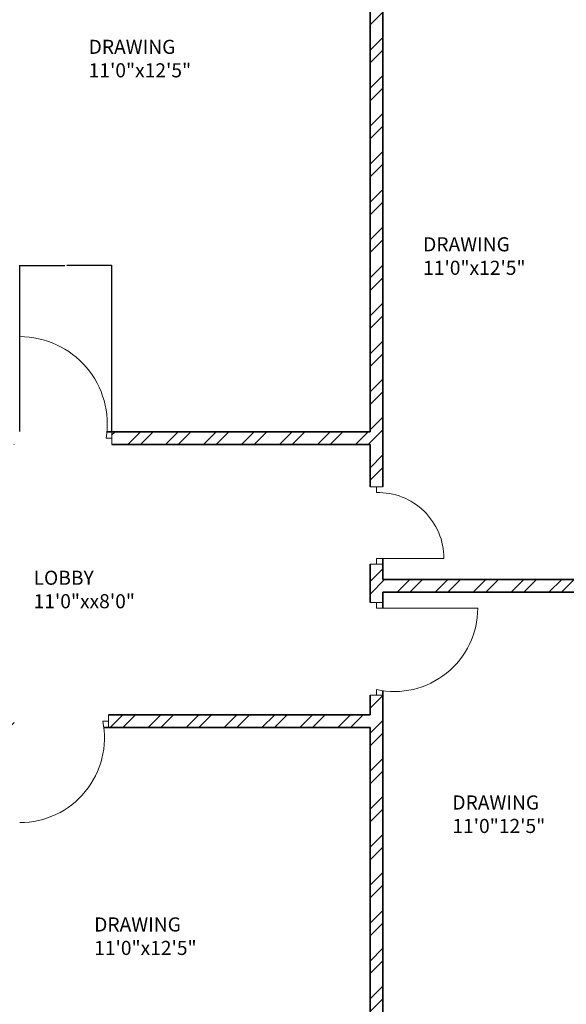
# Model space of a CAD drawing. Units: inches. Extents: x 1962 to 2771, y 1245 to 2660.
# Tile 60 of 114: x 2247 to 2441, y 1831 to 2180. Entities that reach past the tile are written whole.
import ezdxf

# ---------------------------------------------------------------- set-up
doc = ezdxf.new("R2010")
doc.units = ezdxf.units.IN
for name, color, linetype, lineweight in [('A-ANNO-DIMS', 2, 'Continuous', 18), ('A-AREA-IDEN', 7, 'Continuous', 18), ('A-DOOR', 3, 'Continuous', 18), ('A-WALL', 7, 'Continuous', 35), ('A-WALL-PATT', 252, 'Continuous', 13)]:
    doc.layers.add(name, color=color, linetype=linetype, lineweight=lineweight)
doc.styles.get("Standard").update_dxf_attribs({"font": 'arial.ttf'})
doc.dimstyles.get("Standard").update_dxf_attribs({"dimtxt": 0.18, "dimasz": 0.18, "dimexe": 0.18, "dimexo": 0.0625, "dimgap": 0.09, "dimtad": 0, "dimtih": 1, "dimtoh": 1, "dimdec": 4, "dimzin": 0, "dimdsep": 46, "dimtxsty": 'Standard', "dimcen": 0.09, "dimadec": 0, "dimazin": 0, "dimtfac": 1, "dimtdec": 4, "dimtofl": 0, "dimtmove": 0, "dimatfit": 3, "dimfxl": 1, "dimtolj": 1, "dimtzin": 0, "dimarcsym": 0})

# ---------------------------------------------------------------- blocks, each defined once
blk = doc.blocks.new('*D40')
at = {"layer": 'A-ANNO-DIMS', "color": 0, "lineweight": -2, "transparency": 16777216}
for p, q in [((2072.02, 2033.91), (2072.02, 2583.47)), ((2072.2, 2583.29), (2366.02, 2583.29)), ((2660.63, 2583.29), (2366.81, 2583.29)), ((2660.81, 2524.41), (2660.81, 2583.47))]:
    blk.add_line(p, q, dxfattribs=at)
at = {"layer": 'A-ANNO-DIMS', "color": 0, "transparency": 16777216}
for points in [[(2072.2, 2583.32), (2072.2, 2583.26), (2072.02, 2583.29)], [(2660.63, 2583.32), (2660.63, 2583.26), (2660.81, 2583.29)]]:
    blk.add_solid(points, dxfattribs=at)
at = {"layer": 'Defpoints', "color": 0, "transparency": 16777216}
for p in [(2660.81, 2583.29), (2660.81, 2524.34), (2072.02, 2033.84)]:
    blk.add_point(p, dxfattribs=at)
at = {"layer": 'A-ANNO-DIMS', "color": 0, "transparency": 16777216, "insert": (2366.41, 2583.29), "char_height": 0.18, "attachment_point": 5}
blk.add_mtext('\\A1;588.8', dxfattribs=at)
blk = doc.blocks.new('*D45')
at = {"layer": 'A-ANNO-DIMS', "color": 0, "lineweight": -2, "transparency": 16777216}
for p, q in [((2246.94, 2033.91), (2246.94, 2092.97)), ((2247.12, 2092.79), (2262.91, 2092.79)), ((2279.48, 2092.79), (2263.69, 2092.79)), ((2279.66, 2033.91), (2279.66, 2092.97))]:
    blk.add_line(p, q, dxfattribs=at)
at = {"layer": 'A-ANNO-DIMS', "color": 0, "transparency": 16777216}
for points in [[(2247.12, 2092.82), (2247.12, 2092.76), (2246.94, 2092.79)], [(2279.48, 2092.82), (2279.48, 2092.76), (2279.66, 2092.79)]]:
    blk.add_solid(points, dxfattribs=at)
at = {"layer": 'Defpoints', "color": 0, "transparency": 16777216}
for p in [(2279.66, 2092.79), (2246.94, 2033.84), (2279.66, 2033.84)]:
    blk.add_point(p, dxfattribs=at)
at = {"layer": 'A-ANNO-DIMS', "color": 0, "transparency": 16777216, "insert": (2263.3, 2092.79), "char_height": 0.18, "attachment_point": 5}
blk.add_mtext('\\A1;32.72', dxfattribs=at)

msp = doc.modelspace()

# ---------------------------------------------------------------- hatches: boundary and pattern name
at = {"layer": 'A-WALL-PATT'}
h = msp.add_hatch(dxfattribs=at)
h.set_pattern_fill('ANSI32', color=256)
h.paths.add_polyline_path([(2090.8074, 2467.3437), (2141.6481, 2467.3437), (2141.6481, 2469.5937), (2141.6481, 2471.8437), (2086.3074, 2471.8437), (2086.3074, 2422.5333), (2090.8074, 2422.5333)])
h.paths.add_polyline_path([(2282.7664, 2471.8437), (2204.8982, 2471.8437), (2204.8982, 2467.3437), (2234.8074, 2467.3437), (2234.8074, 2311.3437), (2228.7492, 2311.3437), (2228.7492, 2306.8437), (2234.8074, 2306.8437), (2331.9227, 2306.8437), (2331.9227, 2309.0937), (2331.9227, 2311.3437), (2239.3074, 2311.3437), (2239.3074, 2467.3437), (2282.7664, 2467.3437), (2282.7664, 2469.5937)])
h.paths.add_polyline_path([(2471.4531, 2519.8437), (2552.011, 2519.8437), (2564.3996, 2519.8437), (2564.3996, 2511.1389), (2568.8996, 2511.1389), (2568.8996, 2524.3437), (2466.9531, 2524.3437), (2466.9531, 2471.8437), (2450.0749, 2471.8437), (2446.4672, 2471.8437), (2446.4672, 2467.3437), (2450.0749, 2467.3437), (2475.9988, 2467.3437), (2475.9988, 2469.5937), (2475.9988, 2471.8437), (2471.4531, 2471.8437)])
h.paths.add_polyline_path([(2575.2231, 2469.5937), (2575.2231, 2471.8437), (2568.8996, 2471.8437), (2568.8996, 2487.1389), (2564.3996, 2487.1389), (2564.3996, 2471.8437), (2556.511, 2471.8437), (2499.2904, 2471.8437), (2499.2904, 2467.3437), (2507.8074, 2467.3437), (2507.8074, 2311.3437), (2414.863, 2311.3437), (2414.863, 2306.8437), (2512.3074, 2306.8437), (2517.0114, 2306.8437), (2517.0114, 2309.0937), (2517.0114, 2311.3437), (2512.3074, 2311.3437), (2512.3074, 2467.3437), (2575.2231, 2467.3437)])
h.paths.add_polyline_path([(2660.8074, 2471.8437), (2600.9602, 2471.8437), (2600.9602, 2467.3437), (2656.3074, 2467.3437), (2656.3074, 2432.5704), (2660.8074, 2432.5704)])
h.paths.add_polyline_path([(2660.8074, 2372.5704), (2656.3074, 2372.5704), (2656.3074, 2311.3437), (2600.276, 2311.3437), (2600.276, 2309.0937), (2600.276, 2306.8437), (2656.3074, 2306.8437), (2656.3074, 2296.2593), (2660.8074, 2296.2593)])
h.paths.add_polyline_path([(2572.3074, 2306.8437), (2577.1385, 2306.8437), (2577.1385, 2311.3437), (2551.082, 2311.3437), (2551.082, 2306.8437), (2567.8074, 2306.8437), (2567.8074, 2258.8437), (2540.0574, 2258.8437), (2540.0574, 2256.5937), (2540.0574, 2254.3437), (2567.8074, 2254.3437), (2656.3074, 2254.3437), (2656.3074, 2236.9085), (2660.8074, 2236.9085), (2660.8074, 2272.2593), (2656.3074, 2272.2593), (2656.3074, 2258.8437), (2572.3074, 2258.8437)])
h.paths.add_polyline_path([(2512.3074, 2254.3437), (2518.8716, 2254.3437), (2518.8716, 2256.5937), (2518.8716, 2258.8437), (2507.8074, 2258.8437), (2507.8074, 2177.8437), (2567.8074, 2177.8437), (2567.8074, 2172.9628), (2572.3074, 2172.9628), (2572.3074, 2177.8437), (2656.3074, 2177.8437), (2656.3074, 2166.4846), (2660.8074, 2166.4846), (2660.8074, 2200.9085), (2656.3074, 2200.9085), (2656.3074, 2182.3437), (2512.3074, 2182.3437)])
h.paths.add_polyline_path([(2656.3074, 2129.8437), (2572.3074, 2129.8437), (2572.3074, 2150.3044), (2570.0574, 2150.3044), (2567.8074, 2150.3044), (2567.8074, 2129.8437), (2507.8074, 2129.8437), (2507.8074, 2116.3027), (2510.0574, 2116.3027), (2512.3074, 2116.3027), (2512.3074, 2125.3437), (2567.8074, 2125.3437), (2572.3074, 2125.3437), (2656.3074, 2125.3437)])
h.paths.add_polyline_path([(2090.8074, 2362.5333), (2086.3074, 2362.5333), (2086.3074, 2298.6242), (2090.8074, 2298.6242), (2090.8074, 2306.8437), (2174.8074, 2306.8437), (2174.8074, 2286.4178), (2179.3074, 2286.4178), (2179.3074, 2306.8437), (2192.8641, 2306.8437), (2192.8641, 2309.0937), (2192.8641, 2311.3437), (2090.8074, 2311.3437)])
h.paths.add_polyline_path([(2209.156, 2258.8437), (2179.3074, 2258.8437), (2179.3074, 2263.2236), (2177.0574, 2263.2236), (2174.8074, 2263.2236), (2174.8074, 2258.8437), (2090.8074, 2258.8437), (2090.8074, 2274.6242), (2086.3074, 2274.6242), (2086.3074, 2238.2967), (2088.5574, 2238.2967), (2090.8074, 2238.2967), (2090.8074, 2254.3437), (2209.156, 2254.3437)])
h.paths.add_polyline_path([(2090.8074, 2177.8437), (2234.8074, 2177.8437), (2234.8074, 2173.1428), (2239.3074, 2173.1428), (2239.3074, 2258.8437), (2230.8442, 2258.8437), (2230.8442, 2256.5937), (2230.8442, 2254.3437), (2234.8074, 2254.3437), (2234.8074, 2182.3437), (2090.8074, 2182.3437), (2090.8074, 2202.2967), (2086.3074, 2202.2967), (2086.3074, 2140.0389), (2090.8074, 2140.0389)])
h.paths.add_polyline_path([(2090.8074, 2080.0389), (2086.3074, 2080.0389), (2086.3074, 2033.8437), (2090.8074, 2033.8437)], flags=17)
h.paths.add_polyline_path([(2244.9405, 2033.8437), (2239.3074, 2033.8437), (2239.3074, 2142.0665), (2237.2592, 2142.0665), (2234.8074, 2142.0665), (2234.8074, 2033.8437), (2090.8074, 2033.8437), (2076.5204, 2033.8437), (2072.0204, 2033.8437), (2072.0204, 2000.4493), (2076.5204, 2000.4493), (2076.5204, 2029.3437), (2090.8074, 2029.3437), (2244.9405, 2029.3437), (2244.9405, 2031.5937)])
h.paths.add_polyline_path([(2234.8074, 1933.3437), (2076.5204, 1933.3437), (2076.5204, 1952.4493), (2074.2704, 1952.4493), (2072.0204, 1952.4493), (2072.0204, 1933.3437), (2072.0204, 1928.8437), (2234.8074, 1928.8437)])
h.paths.add_polyline_path([(2090.8074, 1928.8437), (2086.3074, 1928.8437), (2086.3074, 1906.5013), (2090.8074, 1906.5013)])
h.paths.add_polyline_path([(2090.8074, 1846.5013), (2086.3074, 1846.5013), (2086.3074, 1769.9917), (2088.5574, 1769.9917), (2090.8074, 1769.9917), (2090.8074, 1780.3437), (2234.8074, 1780.3437), (2234.8074, 1708.3437), (2230.3764, 1708.3437), (2230.3764, 1703.8437), (2239.3074, 1703.8437), (2239.3074, 1792.6669), (2237.0574, 1792.6669), (2234.8074, 1792.6669), (2234.8074, 1784.8437), (2090.8074, 1784.8437)])
h.paths.add_polyline_path([(2239.3074, 1928.8437), (2244.9405, 1928.8437), (2244.9405, 1931.0937), (2244.9405, 1933.3437), (2234.8074, 1933.3437), (2234.8074, 1928.8437), (2234.8074, 1825.5949), (2239.3074, 1825.5949)])
h.paths.add_polyline_path([(2148.0425, 1649.0937), (2148.0425, 1651.3437), (2090.8074, 1651.3437), (2090.8074, 1646.8437), (2148.0425, 1646.8437)], flags=0)
h.paths.add_polyline_path([(2207.5601, 1708.3437), (2090.8074, 1708.3437), (2090.8074, 1703.8437), (2174.8074, 1703.8437), (2174.8074, 1651.3437), (2170.4457, 1651.3437), (2170.4457, 1646.8437), (2195.9924, 1646.8437), (2195.9924, 1649.0937), (2195.9924, 1651.3437), (2179.3074, 1651.3437), (2179.3074, 1703.8437), (2207.5601, 1703.8437), (2207.5601, 1706.0937)])
h.paths.add_polyline_path([(2090.8074, 1733.9917), (2086.3074, 1733.9917), (2086.3074, 1696.1032), (2088.5574, 1696.1032), (2090.8074, 1696.1032)])
h.paths.add_polyline_path([(2090.8074, 1672.1032), (2086.3074, 1672.1032), (2086.3074, 1600.3335), (2090.8074, 1600.3335)])
h.paths.add_polyline_path([(2090.8074, 1540.3335), (2086.3074, 1540.3335), (2086.3074, 1486.3437), (2139.6766, 1486.3437), (2139.6766, 1490.8437), (2090.8074, 1490.8437)])
h.paths.add_polyline_path([(2302.3876, 1490.8437), (2239.3074, 1490.8437), (2239.3074, 1646.8437), (2335.9994, 1646.8437), (2335.9994, 1651.3437), (2229.884, 1651.3437), (2229.884, 1646.8437), (2234.8074, 1646.8437), (2234.8074, 1490.8437), (2202.7103, 1490.8437), (2202.7103, 1488.5937), (2202.7103, 1486.3437), (2275.0699, 1486.3437), (2275.0699, 1475.772), (2279.5699, 1475.772), (2279.5699, 1486.3437), (2302.3876, 1486.3437)])
h.paths.add_polyline_path([(2279.5699, 1451.772), (2275.0699, 1451.772), (2275.0699, 1438.3437), (2174.8074, 1438.3437), (2174.8074, 1486.3437), (2179.7922, 1486.3437), (2179.7922, 1490.8437), (2163.3585, 1490.8437), (2163.3585, 1488.5937), (2163.3585, 1486.3437), (2170.3074, 1486.3437), (2170.3074, 1433.8437), (2279.5699, 1433.8437)])
h.paths.add_polyline_path([(2427.2363, 1490.8437), (2375.8074, 1490.8437), (2375.8074, 1646.8437), (2381.6401, 1646.8437), (2381.6401, 1651.3437), (2365.887, 1651.3437), (2365.887, 1649.0937), (2365.887, 1646.8437), (2371.3074, 1646.8437), (2371.3074, 1490.8437), (2327.5627, 1490.8437), (2327.5627, 1488.5937), (2327.5627, 1486.3437), (2371.3074, 1486.3437), (2371.3074, 1433.8437), (2375.8074, 1433.8437), (2375.8074, 1486.3437), (2427.2363, 1486.3437)])
h.paths.add_polyline_path([(2512.3074, 1646.8437), (2519.4351, 1646.8437), (2519.4351, 1649.0937), (2519.4351, 1651.3437), (2507.8074, 1651.3437), (2416.0063, 1651.3437), (2416.0063, 1649.0937), (2416.0063, 1646.8437), (2507.8074, 1646.8437), (2507.8074, 1490.8437), (2497.0532, 1490.8437), (2497.0532, 1488.5937), (2497.0532, 1486.3437), (2574.9344, 1486.3437), (2574.9344, 1476.0181), (2579.4344, 1476.0181), (2579.4344, 1486.3437), (2584.4872, 1486.3437), (2584.3074, 1490.8437), (2512.3074, 1490.8437)])
h.paths.add_polyline_path([(2470.5091, 1486.3437), (2473.9767, 1486.3437), (2473.9767, 1490.8437), (2449.6605, 1490.8437), (2449.6605, 1488.5937), (2449.6605, 1486.3437), (2466.0091, 1486.3437), (2466.0091, 1433.8437), (2470.5091, 1433.8437), (2579.4344, 1433.8437), (2579.4344, 1452.0181), (2574.9344, 1452.0181), (2574.9344, 1438.3437), (2554.5091, 1438.3437), (2470.5091, 1438.3437)])
h.paths.add_polyline_path([(2656.3074, 1490.8437), (2611.86, 1490.8437), (2611.86, 1486.3437), (2656.3074, 1486.3437)])
h.paths.add_polyline_path([(2660.8074, 1532.7007), (2658.5574, 1532.7007), (2656.3074, 1532.7007), (2656.3074, 1486.3437), (2660.8074, 1486.3437)])
h.paths.add_polyline_path([(2660.8074, 1664.9663), (2656.3074, 1664.9663), (2656.3074, 1651.3437), (2602.2313, 1651.3437), (2602.2313, 1646.8437), (2656.3074, 1646.8437), (2656.3074, 1592.7007), (2660.8074, 1592.7007)])
h.paths.add_polyline_path([(2660.8074, 1724.5221), (2656.3074, 1724.5221), (2656.3074, 1703.8437), (2542.4725, 1703.8437), (2542.4725, 1699.3437), (2567.8074, 1699.3437), (2567.8074, 1651.3437), (2552.7766, 1651.3437), (2552.7766, 1649.0937), (2552.7766, 1646.8437), (2577.2878, 1646.8437), (2577.2878, 1649.0937), (2577.2878, 1651.3437), (2572.3074, 1651.3437), (2572.3074, 1699.3437), (2656.3074, 1699.3437), (2656.3074, 1688.9663), (2660.8074, 1688.9663)])
h.paths.add_polyline_path([(2660.8074, 1880.6524), (2656.3074, 1880.6524), (2656.3074, 1832.8437), (2512.3074, 1832.8437), (2512.3074, 1837.8959), (2507.8074, 1837.8959), (2507.8074, 1828.3437), (2567.8074, 1828.3437), (2567.8074, 1804.3437), (2572.3074, 1804.3437), (2572.3074, 1828.3437), (2656.3074, 1828.3437), (2656.3074, 1818.6778), (2660.8074, 1818.6778)])
h.paths.add_polyline_path([(2660.8074, 1794.6778), (2656.3074, 1794.6778), (2656.3074, 1780.3437), (2572.3074, 1780.3437), (2572.3074, 1783.0303), (2570.0574, 1783.0303), (2567.8074, 1783.0303), (2567.8074, 1780.3437), (2507.8074, 1780.3437), (2507.8074, 1699.3437), (2517.8858, 1699.3437), (2517.8858, 1701.5937), (2517.8858, 1703.8437), (2512.3074, 1703.8437), (2512.3074, 1775.8437), (2656.3074, 1775.8437), (2656.3074, 1760.5221), (2660.8074, 1760.5221)])
h.paths.add_polyline_path([(2660.8074, 1981.3437), (2660.8074, 2020.2808), (2658.5574, 2020.2808), (2656.3074, 2020.2808), (2656.3074, 1981.3437), (2512.3074, 1981.3437), (2512.3074, 2086.6996), (2507.8074, 2086.6996), (2507.8074, 1981.3437), (2375.8074, 1981.3437), (2375.8074, 1986.8505), (2373.5574, 1986.8505), (2371.3074, 1986.8505), (2371.3074, 1973.2607), (2375.8074, 1973.2607), (2375.8074, 1976.8437), (2507.8074, 1976.8437), (2507.8074, 1865.4281), (2510.0574, 1865.4281), (2512.3074, 1865.4281), (2512.3074, 1976.8437), (2660.8074, 1976.8437)])
h.paths.add_polyline_path([(2375.8074, 1940.297), (2373.5574, 1940.297), (2371.3074, 1940.297), (2371.3074, 1933.3437), (2278.4434, 1933.3437), (2278.4434, 1928.8437), (2371.3074, 1928.8437), (2371.3074, 1651.3437), (2375.8074, 1651.3437)])
h.paths.add_polyline_path([(2660.8074, 1976.8437), (2656.3074, 1976.8437), (2656.3074, 1940.6524), (2660.8074, 1940.6524)], flags=17)
h.paths.add_polyline_path([(2660.8074, 2142.4846), (2656.3074, 2142.4846), (2656.3074, 2080.2808), (2660.8074, 2080.2808)])
h.paths.add_polyline_path([(2381.4189, 2311.3437), (2375.8074, 2311.3437), (2375.8074, 2467.3437), (2424.7242, 2467.3437), (2424.7242, 2469.5937), (2424.7242, 2471.8437), (2375.8074, 2471.8437), (2375.8074, 2524.3437), (2371.3074, 2524.3437), (2371.3074, 2471.8437), (2307.2097, 2471.8437), (2307.2097, 2467.3437), (2371.3074, 2467.3437), (2371.3074, 2311.3437), (2366.8901, 2311.3437), (2366.8901, 2306.8437), (2371.3074, 2306.8437), (2371.3074, 2033.8437), (2279.6589, 2033.8437), (2279.6589, 2029.3437), (2371.3074, 2029.3437), (2371.3074, 2014.2598), (2375.8074, 2014.2598), (2375.8074, 2306.8437), (2381.4189, 2306.8437)])
h.paths.add_polyline_path([(2263.3074, 2524.3437), (2170.3074, 2524.3437), (2170.3074, 2519.8437), (2170.3074, 2471.8437), (2165.0312, 2471.8437), (2165.0312, 2467.3437), (2179.6721, 2467.3437), (2179.6721, 2469.5161), (2179.6721, 2471.8437), (2174.8074, 2471.8437), (2174.8074, 2519.8437), (2258.8074, 2519.8437), (2258.8074, 2511.6436), (2263.3074, 2511.6436)])
h.paths.add_polyline_path([(2245.0232, 1361.4123), (2492.9468, 1361.4123), (2492.9468, 1398.505), (2245.0232, 1398.505)], flags=9)
h.paths.add_polyline_path([(2388.1434, 2086.6936), (2425.0704, 2086.6936), (2425.0704, 2105.3509), (2388.1434, 2105.3509)], flags=9)
h.paths.add_polyline_path([(2404.922, 2242.6744), (2445.7337, 2242.6744), (2445.7337, 2261.3318), (2404.922, 2261.3318)], flags=9)
h.paths.add_polyline_path([(2269.4107, 2156.7935), (2306.3378, 2156.7935), (2306.3378, 2175.4508), (2269.4107, 2175.4508)], flags=9)
h.paths.add_polyline_path([(2269.3277, 2233.4343), (2306.2547, 2233.4343), (2306.2547, 2252.0917), (2269.3277, 2252.0917)], flags=9)
h.paths.add_polyline_path([(2431.6052, 2320.6922), (2470.4456, 2320.6922), (2470.4456, 2339.3495), (2431.6052, 2339.3495)], flags=25)
h.paths.add_polyline_path([(2249.6902, 2315.7608), (2288.5306, 2315.7608), (2288.5306, 2334.4182), (2249.6902, 2334.4182)], flags=25)
h.paths.add_polyline_path([(2096.9301, 2314.3181), (2135.7704, 2314.3181), (2135.7704, 2332.9755), (2096.9301, 2332.9755)], flags=25)
h.paths.add_polyline_path([(2134.3475, 2285.7089), (2161.4655, 2285.7089), (2161.4655, 2304.3662), (2134.3475, 2304.3662)], flags=9)
h.paths.add_polyline_path([(2126.5155, 2209.4076), (2159.9227, 2209.4076), (2159.9227, 2228.065), (2126.5155, 2228.065)], flags=25)
h.paths.add_polyline_path([(2110.5753, 2141.5299), (2149.4157, 2141.5299), (2149.4157, 2160.1872), (2110.5753, 2160.1872)], flags=25)
h.paths.add_polyline_path([(2249.8618, 1968.3317), (2286.3966, 1968.3317), (2286.3966, 1986.989), (2249.8618, 1986.989)], flags=9)
h.paths.add_polyline_path([(2395.9507, 1777.0051), (2436.7624, 1777.0051), (2436.7624, 1795.6625), (2395.9507, 1795.6625)], flags=9)
h.paths.add_polyline_path([(2398.5259, 1888.5651), (2435.0062, 1888.5651), (2435.0062, 1907.2224), (2398.5259, 1907.2224)], flags=25)
h.paths.add_polyline_path([(2259.3506, 1728.3559), (2296.2776, 1728.3559), (2296.2776, 1747.0132), (2259.3506, 1747.0132)], flags=9)
h.paths.add_polyline_path([(2271.3698, 1845.268), (2308.2968, 1845.268), (2308.2968, 1863.9253), (2271.3698, 1863.9253)], flags=9)
h.paths.add_polyline_path([(2120.9355, 1786.3027), (2159.7759, 1786.3027), (2159.7759, 1804.9601), (2120.9355, 1804.9601)], flags=25)
h.paths.add_polyline_path([(2121.3164, 1732.1043), (2154.7236, 1732.1043), (2154.7236, 1750.7616), (2121.3164, 1750.7616)], flags=25)
h.paths.add_polyline_path([(2118.3706, 1678.8997), (2147.5282, 1678.8997), (2147.5282, 1697.557), (2118.3706, 1697.557)], flags=25)
h.paths.add_polyline_path([(2385.9227, 1493.557), (2424.763, 1493.557), (2424.763, 1512.2143), (2385.9227, 1512.2143)], flags=25)
h.paths.add_polyline_path([(2248.7058, 1500.0256), (2287.5462, 1500.0256), (2287.5462, 1518.6829), (2248.7058, 1518.6829)], flags=25)
h.paths.add_polyline_path([(2104.1669, 1617.3771), (2143.0073, 1617.3771), (2143.0073, 1636.0344), (2104.1669, 1636.0344)], flags=9)
h.paths.add_polyline_path([(2096.0714, 1447.8824), (2137.3845, 1447.8824), (2137.3845, 1458.1859), (2096.0714, 1458.1859)], flags=9)
h.paths.add_polyline_path([(2180.6114, 1440.325), (2209.7689, 1440.325), (2209.7689, 1458.9823), (2180.6114, 1458.9823)], flags=25)
h.paths.add_polyline_path([(2316.1698, 1447.9637), (2357.4829, 1447.9637), (2357.4829, 1458.2673), (2316.1698, 1458.2673)], flags=9)
h.paths.add_polyline_path([(2397.6187, 1447.9637), (2438.9318, 1447.9637), (2438.9318, 1458.2673), (2397.6187, 1458.2673)], flags=9)
h.paths.add_polyline_path([(2473.0778, 1439.5953), (2502.2354, 1439.5953), (2502.2354, 1458.2527), (2473.0778, 1458.2527)], flags=25)
h.paths.add_polyline_path([(2589.7027, 1447.8819), (2631.0158, 1447.8819), (2631.0158, 1458.1855), (2589.7027, 1458.1855)], flags=9)
h.paths.add_polyline_path([(2522.4009, 1497.5285), (2561.2413, 1497.5285), (2561.2413, 1516.1859), (2522.4009, 1516.1859)], flags=25)
h.paths.add_polyline_path([(2579.6565, 1671.3482), (2608.8141, 1671.3482), (2608.8141, 1690.0056), (2579.6565, 1690.0056)], flags=25)
h.paths.add_polyline_path([(2544.7038, 1725.5064), (2578.1111, 1725.5064), (2578.1111, 1744.1637), (2544.7038, 1744.1637)], flags=25)
h.paths.add_polyline_path([(2578.1191, 1807.472), (2607.2766, 1807.472), (2607.2766, 1826.1293), (2578.1191, 1826.1293)], flags=25)
h.paths.add_polyline_path([(2595.0614, 1835.1839), (2633.9018, 1835.1839), (2633.9018, 1853.8413), (2595.0614, 1853.8413)], flags=25)
h.paths.add_polyline_path([(2567.0097, 2097.7035), (2605.8501, 2097.7035), (2605.8501, 2116.3609), (2567.0097, 2116.3609)], flags=9)
h.paths.add_polyline_path([(2586.644, 2134.6454), (2615.8015, 2134.6454), (2615.8015, 2153.3027), (2586.644, 2153.3027)], flags=9)
h.paths.add_polyline_path([(2544.6185, 2212.6783), (2578.0258, 2212.6783), (2578.0258, 2231.3356), (2544.6185, 2231.3356)], flags=25)
h.paths.add_polyline_path([(2577.0273, 2256.9023), (2606.1849, 2256.9023), (2606.1849, 2275.5597), (2577.0273, 2275.5597)], flags=24)
h.paths.add_polyline_path([(2605.2683, 2315.2821), (2644.1087, 2315.2821), (2644.1087, 2333.9395), (2605.2683, 2333.9395)], flags=25)
h.paths.add_polyline_path([(2583.1244, 2496.1815), (2624.4375, 2496.1815), (2624.4375, 2506.4851), (2583.1244, 2506.4851)], flags=9)
h.paths.add_polyline_path([(2474.761, 2497.0823), (2503.9185, 2497.0823), (2503.9185, 2515.7397), (2474.761, 2515.7397)], flags=25)
h.paths.add_polyline_path([(2387.5787, 2494.2563), (2428.902, 2494.2563), (2428.902, 2504.5598), (2387.5787, 2504.5598)], flags=9)
h.paths.add_polyline_path([(2300.1657, 2500.1564), (2341.4788, 2500.1564), (2341.4788, 2510.46), (2300.1657, 2510.46)], flags=25)
h.paths.add_polyline_path([(2176.8589, 2497.5843), (2206.0165, 2497.5843), (2206.0165, 2516.2416), (2176.8589, 2516.2416)], flags=25)
h.paths.add_polyline_path([(2097.4668, 2494.9762), (2138.7799, 2494.9762), (2138.7799, 2505.2798), (2097.4668, 2505.2798)], flags=9)

# ---------------------------------------------------------------- linework, layer by layer
at = {"layer": 'A-DOOR'}
for p, q in [((2279.6589, 2031.5937), (2277.6589, 2031.5937)), ((2279.6589, 2033.8437), (2279.6589, 2029.3437)), ((2279.6589, 2029.3437), (2279.6589, 2031.5937)), ((2371.3074, 2014.2598), (2375.8074, 2014.2598)), ((2375.8074, 2014.2598), (2373.5574, 2014.2598)), ((2373.5574, 2014.2598), (2373.5574, 2012.2598)), ((2373.5574, 1986.8505), (2373.5574, 1988.8505)), ((2373.5574, 1988.8505), (2397.5574, 1988.8505)), ((2375.8074, 1986.8505), (2371.3074, 1986.8505)), ((2371.3074, 1986.8505), (2375.8074, 1986.8505)), ((2375.8074, 1986.8505), (2373.5574, 1986.8505)), ((2371.3074, 1973.2607), (2375.8074, 1973.2607)), ((2375.8074, 1973.2607), (2373.5574, 1973.2607)), ((2373.5574, 1973.2607), (2373.5574, 1971.2607)), ((2373.5574, 1971.2607), (2409.5574, 1971.2607)), ((2371.3074, 1940.297), (2375.8074, 1940.297)), ((2373.5574, 1940.297), (2373.5574, 1942.297)), ((2375.8074, 1940.297), (2373.5574, 1940.297)), ((2278.4434, 1933.3437), (2278.4434, 1928.8437)), ((2278.4434, 1931.0937), (2276.4434, 1931.0937)), ((2278.4434, 1928.8437), (2278.4434, 1931.0937))]:
    msp.add_line(p, q, dxfattribs=at)
for centre, radius, start, end in [((2246.9405, 2036.4879), 31.1058, 350.947523, 90), ((2374.1409, 1988.8505), 23.4165, 0, 91.427891), ((2379.906, 1971.2607), 29.6514, 257.636737, 360), ((2246.9405, 1925.1829), 30.0892, 270, 11.329108)]:
    msp.add_arc(centre, radius, start, end, dxfattribs=at)
at = {"layer": 'A-WALL'}
for p, q in [((2371.3074, 2306.8437), (2371.3074, 2033.8437)), ((2375.8074, 2306.8437), (2375.8074, 2014.2598)), ((2277.9337, 2033.8437), (2371.3074, 2033.8437)), ((2279.6589, 2029.3437), (2371.3074, 2029.3437)), ((2371.3074, 2029.3437), (2371.3074, 2014.2598)), ((2375.8074, 1988.8505), (2375.8074, 1981.3437)), ((2371.3074, 1986.8505), (2371.3074, 1973.2607)), ((2375.8074, 1981.3437), (2507.8074, 1981.3437)), ((2375.8074, 1976.8437), (2375.8074, 1971.2607)), ((2507.8074, 1976.8437), (2375.8074, 1976.8437)), ((2371.3074, 1940.297), (2371.3074, 1933.3437)), ((2375.8074, 1941.894), (2375.8074, 1651.3437)), ((2278.4434, 1933.3437), (2371.3074, 1933.3437)), ((2276.8061, 1928.8437), (2371.3074, 1928.8437)), ((2371.3074, 1928.8437), (2371.3074, 1651.3437))]:
    msp.add_line(p, q, dxfattribs=at)

# ---------------------------------------------------------------- texts
at = {"layer": 'A-AREA-IDEN', "char_height": 5, "attachment_point": 1}
for s, width, insert in [('DRAWING\\P11\'0"x12\'5"', 296.386063, (2271.4213, 2172.9628)), ('DRAWING\\P11\'0"x12\'5"', 266.153433, (2390.1539, 2102.8629)), ('LOBBY\\P11\'0"xx8\'0"', 205.076953, (2251.8724, 1984.5044)), ('DRAWING\\P11\'0"12\'5"', 147.153935, (2400.5365, 1904.7343)), ('DRAWING\\P11\'0"x12\'5"', 294.426973, (2273.3804, 1861.4373))]:
    msp.add_mtext_dynamic_manual_height_columns(s, width=width, gutter_width=12.5, heights=[0], dxfattribs=dict(at, insert=insert))

# ---------------------------------------------------------------- dimensions: what is measured, and where the dimension line sits
at = {"layer": 'A-ANNO-DIMS'}
for base, p1, p2, override, picture, middle in [((2660.8074, 2583.2937), (2072.0204, 2033.8437), (2660.8074, 2524.3437), {"dimdec": 1, "dimlfac": 1, "dimrnd": 0, "dimzin": 0, "dimdsep": 46, "dimlunit": 2}, '*D40', (2366.4139, 2583.2937)), ((2279.6589, 2092.7937), (2246.9405, 2033.8437), (2279.6589, 2033.8437), {"dimdec": 2, "dimlfac": 1, "dimrnd": 0, "dimzin": 0, "dimdsep": 46, "dimlunit": 2}, '*D45', (2263.2997, 2092.7937))]:
    dim = msp.add_linear_dim(base=base, p1=p1, p2=p2, dimstyle='Standard', override=override, dxfattribs=at)
    dim.commit()
    dim.dimension.update_dxf_attribs({"geometry": picture, "text_midpoint": middle})

doc.saveas('drawing.dxf')
